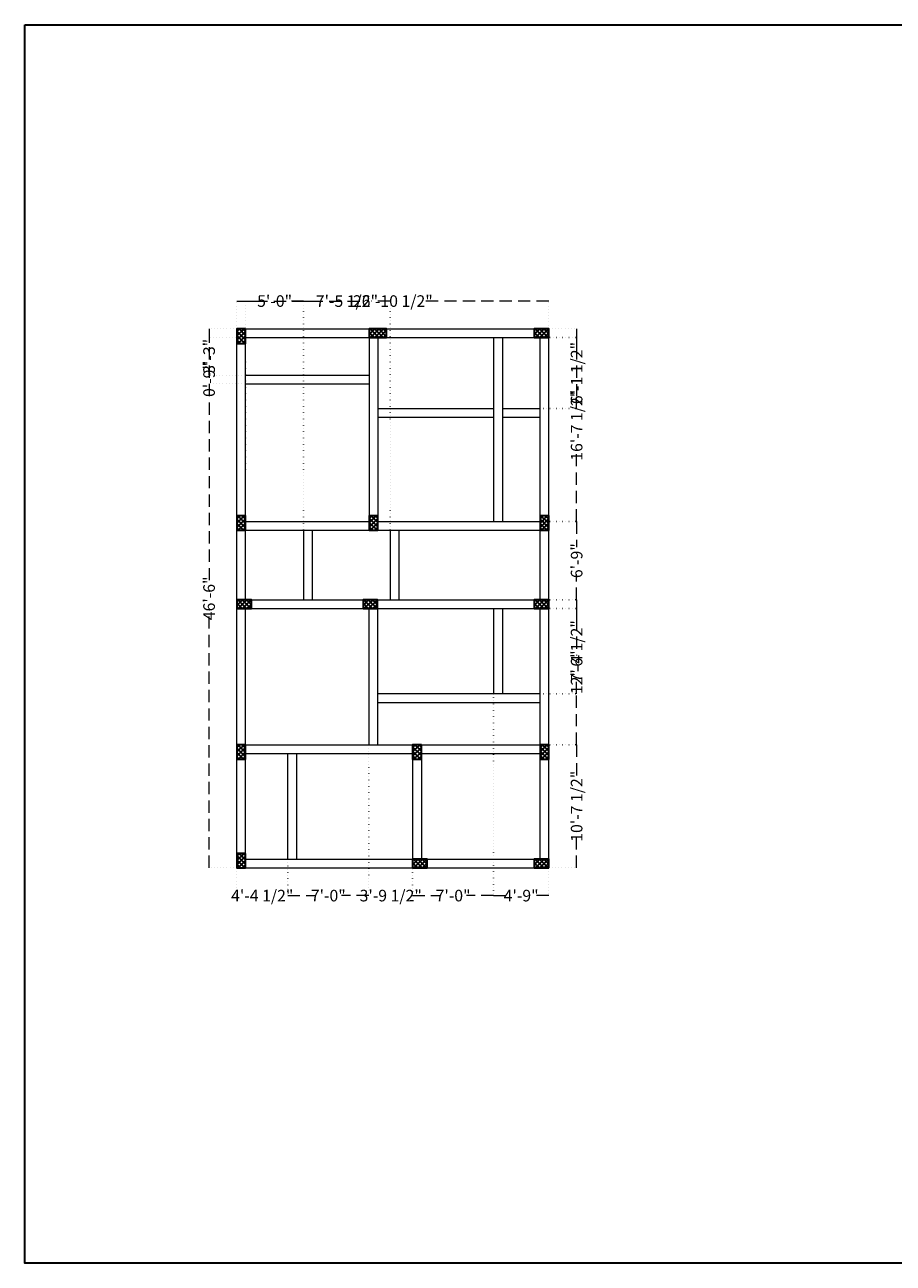
# Model space of a CAD drawing. Units: inches. Extents: x -16911 to -9621, y -48626 to -46270.
# Tile 5 of 20: x -13429 to -12531, y -48626 to -47344. Entities that reach past the tile are written whole.
import ezdxf

# ---------------------------------------------------------------- set-up
doc = ezdxf.new("R2010")
doc.units = ezdxf.units.IN
doc.linetypes.add('DASHED', pattern=[19.05, 12.7, -6.35])
doc.linetypes.add('DOT2', pattern=[3.175, 0, -3.175])
for name, color, linetype, lineweight in [('A-ANNO-DIMS', 2, 'Continuous', 13), ('A-WALL', 7, 'Continuous', 35), ('column', 12, 'Continuous', 30), ('EXT BEAM', 132, 'Continuous', 13), ('S-BEAM', 132, 'Continuous', 25), ('S-COLS', 1, 'Continuous', 30)]:
    doc.layers.add(name, color=color, linetype=linetype, lineweight=lineweight)
doc.styles.add('style9', font='swisscl.ttf', dxfattribs={"height": 12})
doc.dimstyles.new('Dim9', dxfattribs={"dimtxt": 10, "dimasz": 0.199219, "dimexe": 1, "dimexo": 0.5, "dimgap": 1, "dimtad": 0, "dimdec": 1, "dimzin": 0, "dimdsep": 46, "dimlunit": 4, "dimtxsty": 'style9', "dimblk": 'ARCHTICK', "dimcen": 0.09, "dimclrd": 256, "dimclrt": 256, "dimadec": 0, "dimazin": 0, "dimtfac": 1, "dimtdec": 1, "dimtix": 1, "dimtofl": 0, "dimtmove": 1, "dimatfit": 3, "dimfxl": 9, "dimtolj": 1, "dimtzin": 0, "dimlwd": -1, "dimarcsym": 0})

# ---------------------------------------------------------------- blocks, each defined once
blk = doc.blocks.new('TYPICAL BEAMS G-2')
at = {"layer": 'EXT BEAM'}
for p, q in [((-12061.5, -47658.7), (-11738.9, -47658.7)), ((-12061.5, -48216.7), (-12061.5, -47658.7)), ((-11738.9, -48216.7), (-11738.9, -47658.7)), ((-12052.5, -47667.7), (-11924.7, -47667.7)), ((-12052.5, -47939.2), (-12052.5, -47667.7)), ((-11924.7, -47667.7), (-11924.7, -47858.2)), ((-11915.7, -47667.7), (-11747.9, -47667.7)), ((-11915.7, -47667.7), (-11915.7, -47858.2)), ((-11795.9, -47667.7), (-11795.9, -47858.2)), ((-11786.9, -47667.7), (-11786.9, -47858.2)), ((-11747.9, -47858.2), (-11747.9, -47667.7)), ((-12052.5, -47706.7), (-11924.7, -47706.7)), ((-12052.5, -47715.7), (-11924.7, -47715.7)), ((-11915.7, -47741.2), (-11795.9, -47741.2)), ((-11915.7, -47750.2), (-11795.9, -47750.2)), ((-11786.9, -47741.2), (-11747.9, -47741.2)), ((-11786.9, -47750.2), (-11747.9, -47750.2)), ((-12052.5, -47858.2), (-11924.7, -47858.2)), ((-11915.7, -47858.2), (-11747.9, -47858.2)), ((-12052.5, -47867.2), (-11924.7, -47867.2)), ((-11992.5, -47867.2), (-11992.5, -47939.2)), ((-11983.5, -47867.2), (-11983.5, -47939.2)), ((-11915.7, -47867.2), (-11747.9, -47867.2)), ((-11902.9, -47867.2), (-11902.9, -47939.2)), ((-11893.9, -47867.2), (-11893.9, -47939.2)), ((-11747.9, -47939.2), (-11747.9, -47867.2)), ((-12046.5, -47939.2), (-11929.5, -47939.2)), ((-11920.5, -47939.2), (-11738.9, -47939.2)), ((-12052.5, -48089.2), (-12052.5, -47948.2)), ((-12046.5, -47948.2), (-11929.5, -47948.2)), ((-11925, -47948.2), (-11925, -48089.2)), ((-11920.5, -47948.2), (-11738.9, -47948.2)), ((-11916, -47948.2), (-11916, -48089.2)), ((-11795.9, -47948.2), (-11795.9, -48036.7)), ((-11786.9, -47948.2), (-11786.9, -48036.7)), ((-11747.9, -48089.2), (-11747.9, -47948.2)), ((-11747.9, -48036.7), (-11916, -48036.7)), ((-11747.9, -48045.7), (-11916, -48045.7)), ((-12052.5, -48089.2), (-11747.9, -48089.2)), ((-12052.5, -48216.7), (-12052.5, -48098.2)), ((-12052.5, -48098.2), (-11879.7, -48098.2)), ((-12009, -48098.2), (-12009, -48207.7)), ((-12000, -48098.2), (-12000, -48207.7)), ((-11879.7, -48098.2), (-11879.7, -48207.7)), ((-11870.7, -48098.2), (-11747.9, -48098.2)), ((-11870.7, -48098.2), (-11870.7, -48207.7)), ((-11747.9, -48207.7), (-11747.9, -48098.2)), ((-12052.5, -48207.7), (-11879.7, -48207.7)), ((-11870.7, -48207.7), (-11747.9, -48207.7)), ((-12061.5, -48216.7), (-11738.9, -48216.7))]:
    blk.add_line(p, q, dxfattribs=at)
blk = doc.blocks.new('COLUMNS')
at = {"layer": 'column'}
h = blk.add_hatch(dxfattribs=at)
h.set_pattern_fill('ANSI37', color=256, angle=-720)
h.set_pattern_definition([(45, (21703.4588, -104481.6704), (-2.24506403, 2.24506403), []), (135, (21703.4588, -104481.6704), (-2.24506403, -2.24506403), [])])
h.paths.add_polyline_path([(-12061.5, -46401.9), (-12052.5, -46401.9), (-12052.5, -46386.9), (-12061.5, -46386.9)])
h = blk.add_hatch(dxfattribs=at)
h.set_pattern_fill('ANSI37', color=256, angle=-810)
h.set_pattern_definition([(315, (-70004.5392, -80151.7886), (2.24506403, 2.24506403), []), (45, (-70004.5392, -80151.7886), (-2.24506403, 2.24506403), [])])
h.paths.add_polyline_path([(-11924.7, -46386.9), (-11924.7, -46395.9), (-11906.7, -46395.9), (-11906.7, -46386.9)])
h = blk.add_hatch(dxfattribs=at)
h.set_pattern_fill('ANSI37', color=256, angle=-810)
h.set_pattern_definition([(315, (-69833.7395, -80151.7886), (2.24506403, 2.24506403), []), (45, (-69833.7395, -80151.7886), (-2.24506403, 2.24506403), [])])
h.paths.add_polyline_path([(-11753.9, -46386.9), (-11753.9, -46395.9), (-11738.9, -46395.9), (-11738.9, -46386.9)])
h = blk.add_hatch(dxfattribs=at)
h.set_pattern_fill('ANSI37', color=256, angle=-900)
h.set_pattern_definition([(225, (-45817.4075, 11499.4594), (2.24506403, -2.24506403), []), (315, (-45817.4075, 11499.4594), (2.24506403, 2.24506403), [])])
h.paths.add_polyline_path([(-12052.5, -46580.4), (-12061.5, -46580.4), (-12061.5, -46595.4), (-12052.5, -46595.4)])
h = blk.add_hatch(dxfattribs=at)
h.set_pattern_fill('ANSI37', color=256, angle=-720)
h.set_pattern_definition([(45, (21840.2088, -104675.1704), (-2.24506403, 2.24506403), []), (135, (21840.2088, -104675.1704), (-2.24506403, -2.24506403), [])])
h.paths.add_polyline_path([(-11924.7, -46595.4), (-11915.7, -46595.4), (-11915.7, -46580.4), (-11924.7, -46580.4)])
h = blk.add_hatch(dxfattribs=at)
h.set_pattern_fill('ANSI37', color=256, angle=-900)
h.set_pattern_definition([(225, (-45503.8578, 11499.4594), (2.24506403, -2.24506403), []), (315, (-45503.8578, 11499.4594), (2.24506403, 2.24506403), [])])
h.paths.add_polyline_path([(-11738.9, -46580.4), (-11747.9, -46580.4), (-11747.9, -46595.4), (-11738.9, -46595.4)])
h = blk.add_hatch(dxfattribs=at)
h.set_pattern_fill('ANSI37', color=256, angle=-810)
h.set_pattern_definition([(315, (-70141.2892, -80432.2886), (2.24506403, 2.24506403), []), (45, (-70141.2892, -80432.2886), (-2.24506403, 2.24506403), [])])
h.paths.add_polyline_path([(-12061.5, -46667.4), (-12061.5, -46676.4), (-12046.5, -46676.4), (-12046.5, -46667.4)])
h = blk.add_hatch(dxfattribs=at)
h.set_pattern_fill('ANSI37', color=256, angle=-810)
h.set_pattern_definition([(315, (-70010.7892, -80432.2886), (2.24506403, 2.24506403), []), (45, (-70010.7892, -80432.2886), (-2.24506403, 2.24506403), [])])
h.paths.add_polyline_path([(-11931, -46667.4), (-11931, -46676.4), (-11916, -46676.4), (-11916, -46667.4)])
h = blk.add_hatch(dxfattribs=at)
h.set_pattern_fill('ANSI37', color=256, angle=-810)
h.set_pattern_definition([(315, (-69833.7395, -80432.2886), (2.24506403, 2.24506403), []), (45, (-69833.7395, -80432.2886), (-2.24506403, 2.24506403), [])])
h.paths.add_polyline_path([(-11753.9, -46667.4), (-11753.9, -46676.4), (-11738.9, -46676.4), (-11738.9, -46667.4)])
h = blk.add_hatch(dxfattribs=at)
h.set_pattern_fill('ANSI37', color=256, angle=-540)
h.set_pattern_definition([(225, (-45817.4075, 11262.5055), (2.24506403, -2.24506403), []), (315, (-45817.4075, 11262.5055), (2.24506403, 2.24506403), [])])
h.paths.add_polyline_path([(-12052.5, -46817.3), (-12061.5, -46817.3), (-12061.5, -46832.3), (-12052.5, -46832.3)])
h = blk.add_hatch(dxfattribs=at)
h.set_pattern_fill('ANSI37', color=256, angle=-720)
h.set_pattern_definition([(45, (21885.2088, -104912.1242), (-2.24506403, 2.24506403), []), (135, (21885.2088, -104912.1242), (-2.24506403, -2.24506403), [])])
h.paths.add_polyline_path([(-11879.7, -46832.3), (-11870.7, -46832.3), (-11870.7, -46817.3), (-11879.7, -46817.3)])
h = blk.add_hatch(dxfattribs=at)
h.set_pattern_fill('ANSI37', color=256, angle=-720)
h.set_pattern_definition([(45, (22017.1023, -104912.1242), (-2.24506403, 2.24506403), []), (135, (22017.1023, -104912.1242), (-2.24506403, -2.24506403), [])])
h.paths.add_polyline_path([(-11747.8, -46832.3), (-11738.8, -46832.3), (-11738.8, -46817.3), (-11747.8, -46817.3)])
h = blk.add_hatch(dxfattribs=at)
h.set_pattern_fill('ANSI37', color=256, angle=-720)
h.set_pattern_definition([(45, (21703.4588, -105024.6242), (-2.24506403, 2.24506403), []), (135, (21703.4588, -105024.6242), (-2.24506403, -2.24506403), [])])
h.paths.add_polyline_path([(-12061.5, -46944.8), (-12052.5, -46944.8), (-12052.5, -46929.8), (-12061.5, -46929.8)])
h = blk.add_hatch(dxfattribs=at)
h.set_pattern_fill('ANSI37', color=256, angle=-810)
h.set_pattern_definition([(315, (-69959.5392, -80700.7425), (2.24506403, 2.24506403), []), (45, (-69959.5392, -80700.7425), (-2.24506403, 2.24506403), [])])
h.paths.add_polyline_path([(-11879.7, -46935.8), (-11879.7, -46944.8), (-11864.7, -46944.8), (-11864.7, -46935.8)])
h = blk.add_hatch(dxfattribs=at)
h.set_pattern_fill('ANSI37', color=256, angle=-810)
h.set_pattern_definition([(315, (-69833.7395, -80700.7425), (2.24506403, 2.24506403), []), (45, (-69833.7395, -80700.7425), (-2.24506403, 2.24506403), [])])
h.paths.add_polyline_path([(-11753.9, -46935.8), (-11753.9, -46944.8), (-11738.9, -46944.8), (-11738.9, -46935.8)])
at = {"layer": 'column', "ltscale": 0.05}
for points in [[(-12052.5, -46386.9), (-12061.5, -46386.9), (-12061.5, -46401.9), (-12052.5, -46401.9)], [(-11906.7, -46395.9), (-11906.7, -46386.9), (-11924.7, -46386.9), (-11924.7, -46395.9)], [(-11738.9, -46395.9), (-11738.9, -46386.9), (-11753.9, -46386.9), (-11753.9, -46395.9)], [(-12061.5, -46595.4), (-12052.5, -46595.4), (-12052.5, -46580.4), (-12061.5, -46580.4)], [(-11915.7, -46580.4), (-11924.7, -46580.4), (-11924.7, -46595.4), (-11915.7, -46595.4)], [(-11747.9, -46595.4), (-11738.9, -46595.4), (-11738.9, -46580.4), (-11747.9, -46580.4)], [(-12046.5, -46676.4), (-12046.5, -46667.4), (-12061.5, -46667.4), (-12061.5, -46676.4)], [(-11916, -46676.4), (-11916, -46667.4), (-11931, -46667.4), (-11931, -46676.4)], [(-11738.9, -46676.4), (-11738.9, -46667.4), (-11753.9, -46667.4), (-11753.9, -46676.4)], [(-12061.5, -46832.3), (-12052.5, -46832.3), (-12052.5, -46817.3), (-12061.5, -46817.3)], [(-11870.7, -46817.3), (-11879.7, -46817.3), (-11879.7, -46832.3), (-11870.7, -46832.3)], [(-11738.8, -46817.3), (-11747.8, -46817.3), (-11747.8, -46832.3), (-11738.8, -46832.3)], [(-12052.5, -46929.8), (-12061.5, -46929.8), (-12061.5, -46944.8), (-12052.5, -46944.8)], [(-11864.7, -46944.8), (-11864.7, -46935.8), (-11879.7, -46935.8), (-11879.7, -46944.8)], [(-11738.9, -46944.8), (-11738.9, -46935.8), (-11753.9, -46935.8), (-11753.9, -46944.8)]]:
    blk.add_lwpolyline(points, close=True, dxfattribs=at)
blk = doc.blocks.new('_ArchTick')
at = {"color": 0, "linetype": 'ByBlock', "const_width": 0.15}
blk.add_lwpolyline([(-0.5, -0.5), (0.5, 0.5)], dxfattribs=at)
blk = doc.blocks.new('*D89')
at = {"layer": 'A-ANNO-DIMS', "color": 0, "linetype": 'DOT2', "lineweight": -2, "transparency": 16777216}
for p, q in [((-13209.8, -47658.2), (-13209.8, -47629)), ((-12887.3, -47658.2), (-12887.3, -47629))]:
    blk.add_line(p, q, dxfattribs=at)
at = {"layer": 'A-ANNO-DIMS', "linetype": 'DASHED', "transparency": 16777216}
for p, q in [((-13209.8, -47630), (-13081.6, -47630)), ((-12887.3, -47630), (-13015.5, -47630))]:
    blk.add_line(p, q, dxfattribs=at)
at = {"layer": 'Defpoints', "color": 0, "transparency": 16777216}
for p in [(-12887.3, -47630), (-13209.8, -47658.7), (-12887.3, -47658.7)]:
    blk.add_point(p, dxfattribs=at)
at = {"layer": 'A-ANNO-DIMS', "transparency": 16777216, "xscale": 0.19921875, "yscale": 0.19921875, "zscale": 0.19921875, "rotation": 180}
blk.add_blockref('_ArchTick', (-13209.8, -47630), dxfattribs=at)
at = {"layer": 'A-ANNO-DIMS', "transparency": 16777216, "xscale": 0.19921875, "yscale": 0.19921875, "zscale": 0.19921875}
blk.add_blockref('_ArchTick', (-12887.3, -47630), dxfattribs=at)
at = {"layer": 'A-ANNO-DIMS', "transparency": 16777216, "insert": (-13048.5, -47630), "char_height": 12, "attachment_point": 5, "style": 'style9'}
blk.add_mtext('\\A1;26\'-10 1/2"', dxfattribs=at)
blk = doc.blocks.new('*D90')
at = {"layer": 'A-ANNO-DIMS', "color": 0, "linetype": 'DOT2', "lineweight": -2, "transparency": 16777216}
for p, q in [((-13210.3, -47658.7), (-13239.6, -47658.7)), ((-13210.3, -48216.7), (-13239.6, -48216.7))]:
    blk.add_line(p, q, dxfattribs=at)
at = {"layer": 'A-ANNO-DIMS', "linetype": 'DASHED', "transparency": 16777216}
for p, q in [((-13238.6, -47658.7), (-13238.6, -47920.1)), ((-13238.6, -48216.7), (-13238.6, -47955.4))]:
    blk.add_line(p, q, dxfattribs=at)
at = {"layer": 'Defpoints', "color": 0, "transparency": 16777216}
for p in [(-13209.8, -47658.7), (-13238.6, -48216.7), (-13209.8, -48216.7)]:
    blk.add_point(p, dxfattribs=at)
at = {"layer": 'A-ANNO-DIMS', "transparency": 16777216, "xscale": 0.19921875, "yscale": 0.19921875, "zscale": 0.19921875}
for p, rotation in [((-13238.6, -47658.7), 90), ((-13238.6, -48216.7), 270)]:
    blk.add_blockref('_ArchTick', p, dxfattribs=dict(at, rotation=rotation))
at = {"layer": 'A-ANNO-DIMS', "transparency": 16777216, "insert": (-13238.6, -47937.7), "char_height": 12, "attachment_point": 5, "rotation": 90, "style": 'style9'}
blk.add_mtext('\\A1;46\'-6"', dxfattribs=at)
blk = doc.blocks.new('*D91')
at = {"layer": 'A-ANNO-DIMS', "color": 0, "linetype": 'DOT2', "lineweight": -2, "transparency": 16777216}
for p, q in [((-13073.6, -47706.7), (-13239.6, -47706.7)), ((-13073.6, -47715.7), (-13239.6, -47715.7))]:
    blk.add_line(p, q, dxfattribs=at)
at = {"layer": 'A-ANNO-DIMS', "linetype": 'DASHED', "transparency": 16777216}
for p, q in [((-13238.6, -47706.7), (-13238.6, -47706.5)), ((-13238.6, -47715.7), (-13238.6, -47715.9))]:
    blk.add_line(p, q, dxfattribs=at)
at = {"layer": 'Defpoints', "color": 0, "transparency": 16777216}
for p in [(-13073.1, -47706.7), (-13238.6, -47715.7), (-13073.1, -47715.7)]:
    blk.add_point(p, dxfattribs=at)
at = {"layer": 'A-ANNO-DIMS', "transparency": 16777216, "xscale": 0.19921875, "yscale": 0.19921875, "zscale": 0.19921875}
for p, rotation in [((-13238.6, -47706.7), 270), ((-13238.6, -47715.7), 90)]:
    blk.add_blockref('_ArchTick', p, dxfattribs=dict(at, rotation=rotation))
at = {"layer": 'A-ANNO-DIMS', "transparency": 16777216, "insert": (-13238.6, -47711.2), "char_height": 12, "attachment_point": 5, "rotation": 90, "style": 'style9'}
blk.add_mtext('\\A1;0\'-9"', dxfattribs=at)
blk = doc.blocks.new('*D92')
at = {"layer": 'A-ANNO-DIMS', "color": 0, "linetype": 'DOT2', "lineweight": -2, "transparency": 16777216}
for p, q in [((-12886.8, -47658.7), (-12857.4, -47658.7)), ((-12895.8, -47858.2), (-12857.4, -47858.2))]:
    blk.add_line(p, q, dxfattribs=at)
at = {"layer": 'A-ANNO-DIMS', "linetype": 'DASHED', "transparency": 16777216}
for p, q in [((-12858.4, -47658.7), (-12858.4, -47729.4)), ((-12858.4, -47858.2), (-12858.4, -47787.6))]:
    blk.add_line(p, q, dxfattribs=at)
at = {"layer": 'Defpoints', "color": 0, "transparency": 16777216}
for p in [(-12887.3, -47658.7), (-12896.3, -47858.2), (-12858.4, -47858.2)]:
    blk.add_point(p, dxfattribs=at)
at = {"layer": 'A-ANNO-DIMS', "transparency": 16777216, "xscale": 0.19921875, "yscale": 0.19921875, "zscale": 0.19921875}
for p, rotation in [((-12858.4, -47658.7), 90), ((-12858.4, -47858.2), 270)]:
    blk.add_blockref('_ArchTick', p, dxfattribs=dict(at, rotation=rotation))
at = {"layer": 'A-ANNO-DIMS', "transparency": 16777216, "insert": (-12858.4, -47758.5), "char_height": 12, "attachment_point": 5, "rotation": 90, "style": 'style9'}
blk.add_mtext('\\A1;16\'-7 1/2"', dxfattribs=at)
blk = doc.blocks.new('*D93')
at = {"layer": 'A-ANNO-DIMS', "color": 0, "linetype": 'DOT2', "lineweight": -2, "transparency": 16777216}
for p, q in [((-12895.8, -47858.2), (-12857.4, -47858.2)), ((-12895.8, -47939.2), (-12857.4, -47939.2))]:
    blk.add_line(p, q, dxfattribs=at)
at = {"layer": 'A-ANNO-DIMS', "linetype": 'DASHED', "transparency": 16777216}
for p, q in [((-12858.4, -47858.2), (-12858.4, -47884.9)), ((-12858.4, -47939.2), (-12858.4, -47912.6))]:
    blk.add_line(p, q, dxfattribs=at)
at = {"layer": 'Defpoints', "color": 0, "transparency": 16777216}
for p in [(-12896.3, -47858.2), (-12896.3, -47939.2), (-12858.4, -47939.2)]:
    blk.add_point(p, dxfattribs=at)
at = {"layer": 'A-ANNO-DIMS', "transparency": 16777216, "xscale": 0.19921875, "yscale": 0.19921875, "zscale": 0.19921875}
for p, rotation in [((-12858.4, -47858.2), 90), ((-12858.4, -47939.2), 270)]:
    blk.add_blockref('_ArchTick', p, dxfattribs=dict(at, rotation=rotation))
at = {"layer": 'A-ANNO-DIMS', "transparency": 16777216, "insert": (-12858.4, -47898.7), "char_height": 12, "attachment_point": 5, "rotation": 90, "style": 'style9'}
blk.add_mtext('\\A1;6\'-9"', dxfattribs=at)
blk = doc.blocks.new('*D94')
at = {"layer": 'A-ANNO-DIMS', "color": 0, "linetype": 'DOT2', "lineweight": -2, "transparency": 16777216}
for p, q in [((-12895.8, -47939.2), (-12857.4, -47939.2)), ((-12895.8, -48089.2), (-12857.4, -48089.2))]:
    blk.add_line(p, q, dxfattribs=at)
at = {"layer": 'A-ANNO-DIMS', "linetype": 'DASHED', "transparency": 16777216}
for p, q in [((-12858.4, -47939.2), (-12858.4, -47996.8)), ((-12858.4, -48089.2), (-12858.4, -48031.6))]:
    blk.add_line(p, q, dxfattribs=at)
at = {"layer": 'Defpoints', "color": 0, "transparency": 16777216}
for p in [(-12896.3, -47939.2), (-12896.3, -48089.2), (-12858.4, -48089.2)]:
    blk.add_point(p, dxfattribs=at)
at = {"layer": 'A-ANNO-DIMS', "transparency": 16777216, "xscale": 0.19921875, "yscale": 0.19921875, "zscale": 0.19921875}
for p, rotation in [((-12858.4, -47939.2), 90), ((-12858.4, -48089.2), 270)]:
    blk.add_blockref('_ArchTick', p, dxfattribs=dict(at, rotation=rotation))
at = {"layer": 'A-ANNO-DIMS', "transparency": 16777216, "insert": (-12858.4, -48014.2), "char_height": 12, "attachment_point": 5, "rotation": 90, "style": 'style9'}
blk.add_mtext('\\A1;12\'-6"', dxfattribs=at)
blk = doc.blocks.new('*D95')
at = {"layer": 'A-ANNO-DIMS', "color": 0, "linetype": 'DOT2', "lineweight": -2, "transparency": 16777216}
for p, q in [((-12895.8, -48089.2), (-12857.4, -48089.2)), ((-12886.8, -48216.7), (-12857.4, -48216.7))]:
    blk.add_line(p, q, dxfattribs=at)
at = {"layer": 'A-ANNO-DIMS', "linetype": 'DASHED', "transparency": 16777216}
for p, q in [((-12858.4, -48089.2), (-12858.4, -48123.8)), ((-12858.4, -48216.7), (-12858.4, -48182.1))]:
    blk.add_line(p, q, dxfattribs=at)
at = {"layer": 'Defpoints', "color": 0, "transparency": 16777216}
for p in [(-12896.3, -48089.2), (-12887.3, -48216.7), (-12858.4, -48216.7)]:
    blk.add_point(p, dxfattribs=at)
at = {"layer": 'A-ANNO-DIMS', "transparency": 16777216, "xscale": 0.19921875, "yscale": 0.19921875, "zscale": 0.19921875}
for p, rotation in [((-12858.4, -48089.2), 90), ((-12858.4, -48216.7), 270)]:
    blk.add_blockref('_ArchTick', p, dxfattribs=dict(at, rotation=rotation))
at = {"layer": 'A-ANNO-DIMS', "transparency": 16777216, "insert": (-12858.4, -48152.9), "char_height": 12, "attachment_point": 5, "rotation": 90, "style": 'style9'}
blk.add_mtext('\\A1;10\'-7 1/2"', dxfattribs=at)
blk = doc.blocks.new('*D96')
at = {"layer": 'A-ANNO-DIMS', "color": 0, "linetype": 'DOT2', "lineweight": -2, "transparency": 16777216}
for p, q in [((-13201.3, -47667.7), (-13239.6, -47667.7)), ((-13201.3, -47706.7), (-13239.6, -47706.7))]:
    blk.add_line(p, q, dxfattribs=at)
at = {"layer": 'A-ANNO-DIMS', "linetype": 'DASHED', "transparency": 16777216}
for p, q in [((-13238.6, -47667.7), (-13238.6, -47673.4)), ((-13238.6, -47706.7), (-13238.6, -47701))]:
    blk.add_line(p, q, dxfattribs=at)
at = {"layer": 'Defpoints', "color": 0, "transparency": 16777216}
for p in [(-13200.8, -47667.7), (-13238.6, -47706.7), (-13200.8, -47706.7)]:
    blk.add_point(p, dxfattribs=at)
at = {"layer": 'A-ANNO-DIMS', "transparency": 16777216, "xscale": 0.19921875, "yscale": 0.19921875, "zscale": 0.19921875}
for p, rotation in [((-13238.6, -47667.7), 90), ((-13238.6, -47706.7), 270)]:
    blk.add_blockref('_ArchTick', p, dxfattribs=dict(at, rotation=rotation))
at = {"layer": 'A-ANNO-DIMS', "transparency": 16777216, "insert": (-13238.6, -47687.2), "char_height": 12, "attachment_point": 5, "rotation": 90, "style": 'style9'}
blk.add_mtext('\\A1;3\'-3"', dxfattribs=at)
blk = doc.blocks.new('*D97')
at = {"layer": 'A-ANNO-DIMS', "color": 0, "linetype": 'DOT2', "lineweight": -2, "transparency": 16777216}
for p, q in [((-12895.8, -47667.7), (-12857.4, -47667.7)), ((-12895.8, -47741.2), (-12857.4, -47741.2))]:
    blk.add_line(p, q, dxfattribs=at)
at = {"layer": 'A-ANNO-DIMS', "linetype": 'DASHED', "transparency": 16777216}
for p, q in [((-12858.4, -47667.7), (-12858.4, -47679)), ((-12858.4, -47741.2), (-12858.4, -47730))]:
    blk.add_line(p, q, dxfattribs=at)
at = {"layer": 'Defpoints', "color": 0, "transparency": 16777216}
for p in [(-12896.3, -47667.7), (-12896.3, -47741.2), (-12858.4, -47741.2)]:
    blk.add_point(p, dxfattribs=at)
at = {"layer": 'A-ANNO-DIMS', "transparency": 16777216, "xscale": 0.19921875, "yscale": 0.19921875, "zscale": 0.19921875}
for p, rotation in [((-12858.4, -47667.7), 90), ((-12858.4, -47741.2), 270)]:
    blk.add_blockref('_ArchTick', p, dxfattribs=dict(at, rotation=rotation))
at = {"layer": 'A-ANNO-DIMS', "transparency": 16777216, "insert": (-12858.4, -47704.5), "char_height": 12, "attachment_point": 5, "rotation": 90, "style": 'style9'}
blk.add_mtext('\\A1;6\'-1 1/2"', dxfattribs=at)
blk = doc.blocks.new('*D98')
at = {"layer": 'A-ANNO-DIMS', "color": 0, "linetype": 'DOT2', "lineweight": -2, "transparency": 16777216}
for p, q in [((-12895.8, -47948.2), (-12857.4, -47948.2)), ((-12895.8, -48036.7), (-12857.4, -48036.7))]:
    blk.add_line(p, q, dxfattribs=at)
at = {"layer": 'A-ANNO-DIMS', "linetype": 'DASHED', "transparency": 16777216}
for p, q in [((-12858.4, -47948.2), (-12858.4, -47967)), ((-12858.4, -48036.7), (-12858.4, -48017.9))]:
    blk.add_line(p, q, dxfattribs=at)
at = {"layer": 'Defpoints', "color": 0, "transparency": 16777216}
for p in [(-12896.3, -47948.2), (-12896.3, -48036.7), (-12858.4, -48036.7)]:
    blk.add_point(p, dxfattribs=at)
at = {"layer": 'A-ANNO-DIMS', "transparency": 16777216, "xscale": 0.19921875, "yscale": 0.19921875, "zscale": 0.19921875}
for p, rotation in [((-12858.4, -47948.2), 90), ((-12858.4, -48036.7), 270)]:
    blk.add_blockref('_ArchTick', p, dxfattribs=dict(at, rotation=rotation))
at = {"layer": 'A-ANNO-DIMS', "transparency": 16777216, "insert": (-12858.4, -47992.5), "char_height": 12, "attachment_point": 5, "rotation": 90, "style": 'style9'}
blk.add_mtext('\\A1;7\'-4 1/2"', dxfattribs=at)
blk = doc.blocks.new('*D99')
at = {"layer": 'A-ANNO-DIMS', "color": 0, "linetype": 'DOT2', "lineweight": -2, "transparency": 16777216}
for p, q in [((-13157.3, -48208.2), (-13157.3, -48246.4)), ((-13209.8, -48217.2), (-13209.8, -48246.4))]:
    blk.add_line(p, q, dxfattribs=at)
at = {"layer": 'A-ANNO-DIMS', "linetype": 'DASHED', "transparency": 16777216}
for p, q in [((-13209.8, -48245.4), (-13210, -48245.4)), ((-13157.3, -48245.4), (-13157.1, -48245.4))]:
    blk.add_line(p, q, dxfattribs=at)
at = {"layer": 'Defpoints', "color": 0, "transparency": 16777216}
for p in [(-13157.3, -48207.7), (-13209.8, -48216.7), (-13157.3, -48245.4)]:
    blk.add_point(p, dxfattribs=at)
at = {"layer": 'A-ANNO-DIMS', "transparency": 16777216, "xscale": 0.19921875, "yscale": 0.19921875, "zscale": 0.19921875}
blk.add_blockref('_ArchTick', (-13209.8, -48245.4), dxfattribs=at)
at = {"layer": 'A-ANNO-DIMS', "transparency": 16777216, "xscale": 0.19921875, "yscale": 0.19921875, "zscale": 0.19921875, "rotation": 180}
blk.add_blockref('_ArchTick', (-13157.3, -48245.4), dxfattribs=at)
at = {"layer": 'A-ANNO-DIMS', "transparency": 16777216, "insert": (-13183.6, -48245.4), "char_height": 12, "attachment_point": 5, "style": 'style9'}
blk.add_mtext('\\A1;4\'-4 1/2"', dxfattribs=at)
blk = doc.blocks.new('*D100')
at = {"layer": 'A-ANNO-DIMS', "color": 0, "linetype": 'DOT2', "lineweight": -2, "transparency": 16777216}
for p, q in [((-13073.3, -48089.7), (-13073.3, -48246.4)), ((-13157.3, -48208.2), (-13157.3, -48246.4))]:
    blk.add_line(p, q, dxfattribs=at)
at = {"layer": 'A-ANNO-DIMS', "linetype": 'DASHED', "transparency": 16777216}
for p, q in [((-13157.3, -48245.4), (-13129.1, -48245.4)), ((-13073.3, -48245.4), (-13101.6, -48245.4))]:
    blk.add_line(p, q, dxfattribs=at)
at = {"layer": 'Defpoints', "color": 0, "transparency": 16777216}
for p in [(-13073.3, -48089.2), (-13157.3, -48207.7), (-13073.3, -48245.4)]:
    blk.add_point(p, dxfattribs=at)
at = {"layer": 'A-ANNO-DIMS', "transparency": 16777216, "xscale": 0.19921875, "yscale": 0.19921875, "zscale": 0.19921875, "rotation": 180}
blk.add_blockref('_ArchTick', (-13157.3, -48245.4), dxfattribs=at)
at = {"layer": 'A-ANNO-DIMS', "transparency": 16777216, "xscale": 0.19921875, "yscale": 0.19921875, "zscale": 0.19921875}
blk.add_blockref('_ArchTick', (-13073.3, -48245.4), dxfattribs=at)
at = {"layer": 'A-ANNO-DIMS', "transparency": 16777216, "insert": (-13115.3, -48245.4), "char_height": 12, "attachment_point": 5, "style": 'style9'}
blk.add_mtext('\\A1;7\'-0"', dxfattribs=at)
blk = doc.blocks.new('*D101')
at = {"layer": 'A-ANNO-DIMS', "color": 0, "linetype": 'DOT2', "lineweight": -2, "transparency": 16777216}
for p, q in [((-13073.3, -48089.7), (-13073.3, -48246.4)), ((-13028.1, -48208.2), (-13028.1, -48246.4))]:
    blk.add_line(p, q, dxfattribs=at)
at = {"layer": 'A-ANNO-DIMS', "linetype": 'DASHED', "transparency": 16777216}
for p, q in [((-13073.3, -48245.4), (-13073.5, -48245.4)), ((-13028.1, -48245.4), (-13027.9, -48245.4))]:
    blk.add_line(p, q, dxfattribs=at)
at = {"layer": 'Defpoints', "color": 0, "transparency": 16777216}
for p in [(-13073.3, -48089.2), (-13028.1, -48207.7), (-13028.1, -48245.4)]:
    blk.add_point(p, dxfattribs=at)
at = {"layer": 'A-ANNO-DIMS', "transparency": 16777216, "xscale": 0.19921875, "yscale": 0.19921875, "zscale": 0.19921875}
blk.add_blockref('_ArchTick', (-13073.3, -48245.4), dxfattribs=at)
at = {"layer": 'A-ANNO-DIMS', "transparency": 16777216, "xscale": 0.19921875, "yscale": 0.19921875, "zscale": 0.19921875, "rotation": 180}
blk.add_blockref('_ArchTick', (-13028.1, -48245.4), dxfattribs=at)
at = {"layer": 'A-ANNO-DIMS', "transparency": 16777216, "insert": (-13050.7, -48245.4), "char_height": 12, "attachment_point": 5, "style": 'style9'}
blk.add_mtext('\\A1;3\'-9 1/2"', dxfattribs=at)
blk = doc.blocks.new('*D102')
at = {"layer": 'A-ANNO-DIMS', "color": 0, "linetype": 'DOT2', "lineweight": -2, "transparency": 16777216}
for p, q in [((-12944.3, -48037.2), (-12944.3, -48246.4)), ((-13028.1, -48208.2), (-13028.1, -48246.4))]:
    blk.add_line(p, q, dxfattribs=at)
at = {"layer": 'A-ANNO-DIMS', "linetype": 'DASHED', "transparency": 16777216}
for p, q in [((-13028.1, -48245.4), (-12999.9, -48245.4)), ((-12944.3, -48245.4), (-12972.4, -48245.4))]:
    blk.add_line(p, q, dxfattribs=at)
at = {"layer": 'Defpoints', "color": 0, "transparency": 16777216}
for p in [(-12944.3, -48036.7), (-13028.1, -48207.7), (-12944.3, -48245.4)]:
    blk.add_point(p, dxfattribs=at)
at = {"layer": 'A-ANNO-DIMS', "transparency": 16777216, "xscale": 0.19921875, "yscale": 0.19921875, "zscale": 0.19921875, "rotation": 180}
blk.add_blockref('_ArchTick', (-13028.1, -48245.4), dxfattribs=at)
at = {"layer": 'A-ANNO-DIMS', "transparency": 16777216, "xscale": 0.19921875, "yscale": 0.19921875, "zscale": 0.19921875}
blk.add_blockref('_ArchTick', (-12944.3, -48245.4), dxfattribs=at)
at = {"layer": 'A-ANNO-DIMS', "transparency": 16777216, "insert": (-12986.2, -48245.4), "char_height": 12, "attachment_point": 5, "style": 'style9'}
blk.add_mtext('\\A1;7\'-0"', dxfattribs=at)
blk = doc.blocks.new('*D103')
at = {"layer": 'A-ANNO-DIMS', "color": 0, "linetype": 'DOT2', "lineweight": -2, "transparency": 16777216}
for p, q in [((-12944.3, -48037.2), (-12944.3, -48246.4)), ((-12887.3, -48217.2), (-12887.3, -48246.4))]:
    blk.add_line(p, q, dxfattribs=at)
at = {"layer": 'A-ANNO-DIMS', "linetype": 'DASHED', "transparency": 16777216}
for p, q in [((-12944.3, -48245.4), (-12929.6, -48245.4)), ((-12887.3, -48245.4), (-12901.9, -48245.4))]:
    blk.add_line(p, q, dxfattribs=at)
at = {"layer": 'Defpoints', "color": 0, "transparency": 16777216}
for p in [(-12944.3, -48036.7), (-12887.3, -48216.7), (-12887.3, -48245.4)]:
    blk.add_point(p, dxfattribs=at)
at = {"layer": 'A-ANNO-DIMS', "transparency": 16777216, "xscale": 0.19921875, "yscale": 0.19921875, "zscale": 0.19921875, "rotation": 180}
blk.add_blockref('_ArchTick', (-12944.3, -48245.4), dxfattribs=at)
at = {"layer": 'A-ANNO-DIMS', "transparency": 16777216, "xscale": 0.19921875, "yscale": 0.19921875, "zscale": 0.19921875}
blk.add_blockref('_ArchTick', (-12887.3, -48245.4), dxfattribs=at)
at = {"layer": 'A-ANNO-DIMS', "transparency": 16777216, "insert": (-12915.8, -48245.4), "char_height": 12, "attachment_point": 5, "style": 'style9'}
blk.add_mtext('\\A1;4\'-9"', dxfattribs=at)
blk = doc.blocks.new('*D104')
at = {"layer": 'A-ANNO-DIMS', "color": 0, "linetype": 'DOT2', "lineweight": -2, "transparency": 16777216}
for p, q in [((-13200.818183, -47866.74198), (-13200.818183, -47628.99198)), ((-13140.818183, -47866.74198), (-13140.818183, -47628.99198))]:
    blk.add_line(p, q, dxfattribs=at)
at = {"layer": 'A-ANNO-DIMS', "linetype": 'DASHED', "transparency": 16777216}
for p, q in [((-13200.818183, -47629.99198), (-13184.62028, -47629.99198)), ((-13140.818183, -47629.99198), (-13157.016086, -47629.99198))]:
    blk.add_line(p, q, dxfattribs=at)
at = {"layer": 'Defpoints', "color": 0, "transparency": 16777216}
for p in [(-13140.818183, -47629.99198), (-13200.818183, -47867.24198), (-13140.818183, -47867.24198)]:
    blk.add_point(p, dxfattribs=at)
at = {"layer": 'A-ANNO-DIMS', "transparency": 16777216, "xscale": 0.19921875, "yscale": 0.19921875, "zscale": 0.19921875, "rotation": 180}
blk.add_blockref('_ArchTick', (-13200.818183, -47629.99198), dxfattribs=at)
at = {"layer": 'A-ANNO-DIMS', "transparency": 16777216, "xscale": 0.19921875, "yscale": 0.19921875, "zscale": 0.19921875}
blk.add_blockref('_ArchTick', (-13140.818183, -47629.99198), dxfattribs=at)
at = {"layer": 'A-ANNO-DIMS', "transparency": 16777216, "insert": (-13170.818183, -47629.99198), "char_height": 12, "attachment_point": 5, "style": 'style9'}
blk.add_mtext('\\A1;5\'-0"', dxfattribs=at)
blk = doc.blocks.new('*D105')
at = {"layer": 'A-ANNO-DIMS', "color": 0, "linetype": 'DOT2', "lineweight": -2, "transparency": 16777216}
for p, q in [((-13140.8, -47866.7), (-13140.8, -47629)), ((-13051.3, -47866.7), (-13051.3, -47629))]:
    blk.add_line(p, q, dxfattribs=at)
at = {"layer": 'A-ANNO-DIMS', "linetype": 'DASHED', "transparency": 16777216}
for p, q in [((-13140.8, -47630), (-13121.5, -47630)), ((-13051.3, -47630), (-13070.6, -47630))]:
    blk.add_line(p, q, dxfattribs=at)
at = {"layer": 'Defpoints', "color": 0, "transparency": 16777216}
for p in [(-13051.3, -47630), (-13140.8, -47867.2), (-13051.3, -47867.2)]:
    blk.add_point(p, dxfattribs=at)
at = {"layer": 'A-ANNO-DIMS', "transparency": 16777216, "xscale": 0.19921875, "yscale": 0.19921875, "zscale": 0.19921875, "rotation": 180}
blk.add_blockref('_ArchTick', (-13140.8, -47630), dxfattribs=at)
at = {"layer": 'A-ANNO-DIMS', "transparency": 16777216, "xscale": 0.19921875, "yscale": 0.19921875, "zscale": 0.19921875}
blk.add_blockref('_ArchTick', (-13051.3, -47630), dxfattribs=at)
at = {"layer": 'A-ANNO-DIMS', "transparency": 16777216, "insert": (-13096, -47630), "char_height": 12, "attachment_point": 5, "style": 'style9'}
blk.add_mtext('\\A1;7\'-5 1/2"', dxfattribs=at)

msp = doc.modelspace()

# ---------------------------------------------------------------- linework, layer by layer
at = {"layer": 'A-WALL'}
msp.add_lwpolyline([(-13429.245, -47344.007), (-9756.987, -47344.007), (-9756.987, -48625.922), (-13429.245, -48625.922)], close=True, dxfattribs=at)

# ---------------------------------------------------------------- block references
at = {"layer": 'S-BEAM'}
msp.add_blockref('TYPICAL BEAMS G-2', (-1148.344, 0), dxfattribs=at)
at = {"layer": 'S-COLS'}
msp.add_blockref('COLUMNS', (-1148.344, -1271.886), dxfattribs=at)

# ---------------------------------------------------------------- dimensions: what is measured, and where the dimension line sits
at = {"layer": 'A-ANNO-DIMS'}
for base, p1, p2, picture, middle in [((-12887.269, -47629.992), (-13209.818, -47658.742), (-12887.269, -47658.742), '*D89', (-13048.543, -47629.992)), ((-13140.818, -47629.992), (-13200.818, -47867.242), (-13140.818, -47867.242), '*D104', (-13170.818, -47629.992)), ((-13051.269, -47629.992), (-13140.818, -47867.242), (-13051.269, -47867.242), '*D105', (-13096.043, -47629.992)), ((-12944.269, -48245.446), (-13028.068, -48207.696), (-12944.269, -48036.696), '*D102', (-12986.168, -48245.446)), ((-12887.269, -48245.446), (-12944.269, -48036.696), (-12887.269, -48216.696), '*D103', (-12915.769, -48245.446)), ((-13073.318, -48245.446), (-13157.318, -48207.696), (-13073.318, -48089.196), '*D100', (-13115.318, -48245.446)), ((-13028.068183, -48245.445841), (-13073.318183, -48089.195841), (-13028.068183, -48207.695841), '*D101', (-13050.693183, -48245.445841)), ((-13157.318, -48245.446), (-13209.818, -48216.696), (-13157.318, -48207.696), '*D99', (-13183.568, -48245.446))]:
    dim = msp.add_linear_dim(base=base, p1=p1, p2=p2, dimstyle='Dim9', override={"dimdec": 1, "dimlfac": 1, "dimrnd": 0, "dimzin": 1, "dimdsep": 46, "dimlunit": 4, "dimfrac": 2}, dxfattribs=at)
    dim.commit()
    dim.dimension.update_dxf_attribs({"geometry": picture, "text_midpoint": middle})
for base, p1, p2, picture, middle in [((-13238.568, -48216.696), (-13209.818, -47658.742), (-13209.818, -48216.696), '*D90', (-13238.568, -47937.719)), ((-12858.425, -47858.242), (-12887.269, -47658.742), (-12896.269, -47858.242), '*D92', (-12858.425, -47758.492)), ((-13238.568, -47706.742), (-13200.818, -47667.742), (-13200.818, -47706.742), '*D96', (-13238.568, -47687.242)), ((-12858.425, -47741.242), (-12896.269, -47667.742), (-12896.269, -47741.242), '*D97', (-12858.425, -47704.492)), ((-13238.568, -47715.742), (-13073.068, -47706.742), (-13073.068, -47715.742), '*D91', (-13238.568, -47711.242)), ((-12858.425, -47939.242), (-12896.269, -47858.242), (-12896.269, -47939.242), '*D93', (-12858.425, -47898.742)), ((-12858.425, -48089.196), (-12896.269, -47939.242), (-12896.269, -48089.196), '*D94', (-12858.425, -48014.219)), ((-12858.425, -48036.696), (-12896.269, -47948.242), (-12896.269, -48036.696), '*D98', (-12858.425, -47992.469)), ((-12858.425, -48216.696), (-12896.269, -48089.196), (-12887.269, -48216.696), '*D95', (-12858.425, -48152.946))]:
    dim = msp.add_linear_dim(base=base, p1=p1, p2=p2, angle=90, dimstyle='Dim9', override={"dimdec": 1, "dimlfac": 1, "dimrnd": 0, "dimzin": 1, "dimdsep": 46, "dimlunit": 4, "dimfrac": 2}, dxfattribs=at)
    dim.commit()
    dim.dimension.update_dxf_attribs({"geometry": picture, "text_midpoint": middle})

doc.saveas('drawing.dxf')
